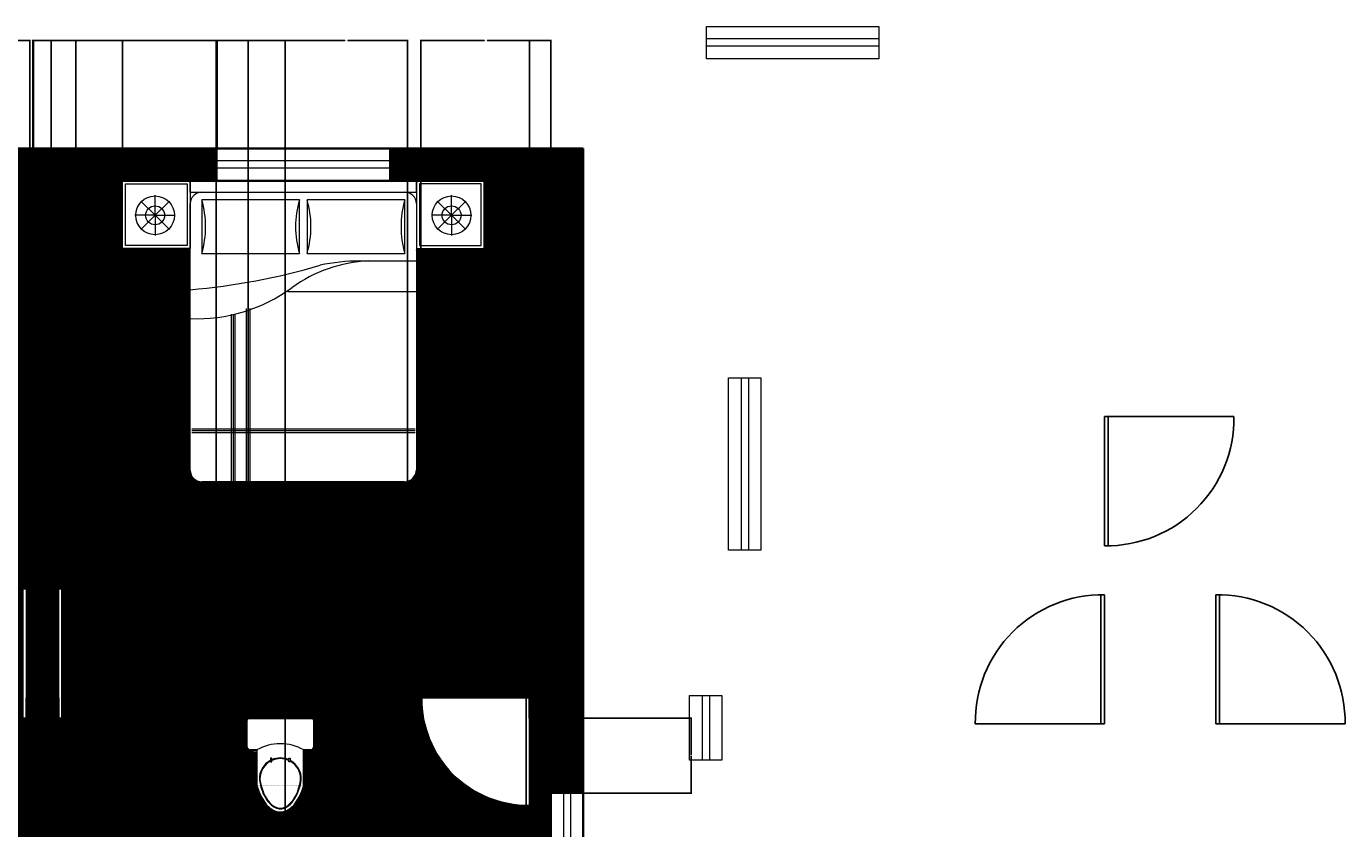
# Model space of a CAD drawing. Units: inches. Extents: x 205 to 1667, y -23 to 828.
# Tile 8 of 10: x 619 to 987, y 418 to 642. Entities that reach past the tile are written whole.
import ezdxf

# ---------------------------------------------------------------- set-up
doc = ezdxf.new("R2010")
doc.units = ezdxf.units.IN
doc.header["$MEASUREMENT"] = 0
for name, color, linetype, lineweight in [('A-ANNO-DIMS', 2, 'Continuous', 18), ('A-AREA-IDEN', 7, 'Continuous', 25), ('A-DOOR', 4, 'Continuous', 25), ('A-FLOR-FIXT', 9, 'Continuous', 18), ('A-FURN', 8, 'Continuous', 18), ('A-GLAZ', 4, 'Continuous', 18), ('A-WALL', 7, 'Continuous', 35)]:
    doc.layers.add(name, color=color, linetype=linetype, lineweight=lineweight)
doc.layers.add('A-FLOR-PATT', color=9, linetype='Continuous', lineweight=9, true_color=0xc7c8ca)
doc.styles.get("Standard").update_dxf_attribs({"font": 'arial.ttf'})
doc.dimstyles.get("Standard").update_dxf_attribs({"dimtxt": 0.18, "dimasz": 0.18, "dimexe": 0.18, "dimexo": 0.0625, "dimgap": 0.09, "dimtad": 0, "dimtih": 1, "dimtoh": 1, "dimdec": 4, "dimzin": 0, "dimdsep": 46, "dimtxsty": 'Standard', "dimcen": 0.09, "dimadec": 0, "dimazin": 0, "dimtfac": 1, "dimtdec": 4, "dimtofl": 0, "dimtmove": 0, "dimatfit": 3, "dimfxl": 1, "dimtolj": 1, "dimtzin": 0, "dimarcsym": 0})

# ---------------------------------------------------------------- blocks, each defined once
blk = doc.blocks.new('A$C068671E6')
for p, q in [((0, 1.5502), (0, 2.0002)), ((0, 2.0002), (0.45, 2.0002)), ((0.02, 1.5702), (0.02, 1.9802)), ((0.02, 1.9802), (0.43, 1.9802)), ((0.43, 1.9802), (0.43, 1.5702)), ((0.45, 2.0002), (0.45, 1.5502)), ((1.9506, 2.0002), (1.9506, 1.5502)), ((2.4006, 2.0002), (1.9506, 2.0002)), ((1.9706, 1.9802), (1.9706, 1.5702)), ((2.3806, 1.9802), (1.9706, 1.9802)), ((2.3806, 1.5702), (2.3806, 1.9802)), ((2.4006, 1.5502), (2.4006, 2.0002)), ((0.216, 1.7702), (0.121, 1.8652)), ((0.216, 1.7702), (0.216, 1.9046)), ((0.216, 1.7702), (0.3111, 1.8652)), ((2.1846, 1.7702), (2.0895, 1.8652)), ((2.1846, 1.7702), (2.1846, 1.9046)), ((2.1846, 1.7702), (2.2796, 1.8652)), ((0.216, 1.7702), (0.0817, 1.7702)), ((0.216, 1.7702), (0.121, 1.6752)), ((0.216, 1.7702), (0.216, 1.6358)), ((0.216, 1.7702), (0.3111, 1.6752)), ((0.216, 1.7702), (0.3504, 1.7702)), ((2.1846, 1.7702), (2.0502, 1.7702)), ((2.1846, 1.7702), (2.0895, 1.6752)), ((2.1846, 1.7702), (2.1846, 1.6358)), ((2.1846, 1.7702), (2.3189, 1.7702)), ((2.1846, 1.7702), (2.2796, 1.6752)), ((0.45, 1.5502), (0, 1.5502)), ((0.43, 1.5702), (0.02, 1.5702)), ((1.9506, 1.5502), (2.4006, 1.5502)), ((1.9706, 1.5702), (2.3806, 1.5702)), ((0.8202, 1.1507), (0.8202, 0)), ((0.8322, 1.1507), (0.8322, 0)), ((0.8442, 1.1507), (0.8442, 0)), ((0.722, 1.1146), (0.722, 0)), ((0.734, 1.1146), (0.734, 0)), ((0.746, 1.1146), (0.746, 0)), ((0.4599, 0.3521), (1.9437, 0.3521)), ((0.4599, 0.3401), (1.9437, 0.3401)), ((0.4599, 0.3281), (1.9437, 0.3281))]:
    blk.add_line(p, q)
at = {"linetype": 'ByBlock'}
for p, q in [((0.45, 1.924), (0.45, 2.0002)), ((0.45, 2.0002), (1.9506, 2.0002)), ((1.9506, 1.924), (1.9506, 2.0002)), ((0.45, 1.924), (1.9506, 1.924)), ((0.45, 0.0762), (0.45, 1.8478)), ((1.1744, 1.8732), (0.5262, 1.8732)), ((0.5262, 1.8732), (0.5262, 1.5176)), ((1.1744, 1.5176), (1.1744, 1.8732)), ((1.8744, 1.8732), (1.2252, 1.8732)), ((1.2252, 1.8732), (1.2252, 1.5176)), ((1.8744, 1.5176), (1.8744, 1.8732)), ((1.9506, 1.8478), (1.9506, 0.08)), ((0.5262, 1.5176), (1.1744, 1.5176)), ((1.2252, 1.5176), (1.8744, 1.5176)), ((1.5747, 1.4668), (1.9506, 1.4668)), ((1.0982, 1.2636), (1.9506, 1.2636)), ((1.8706, 0), (0.5262, 0))]:
    blk.add_line(p, q, dxfattribs=at)
for centre, radius in [((0.216, 1.7702), 0.1285), ((2.1846, 1.7702), 0.1285), ((0.216, 1.7702), 0.0628), ((2.1846, 1.7702), 0.0628)]:
    blk.add_circle(centre, radius)
for centre, radius, start, end in [((0.5262, 1.8478), 0.0762, 90, 180), ((-0.0834, 1.6954), 0.635, 343.73979, 16.26021), ((1.784, 1.6954), 0.635, 163.73979, 196.26021), ((0.6156, 1.6954), 0.635, 343.73979, 16.26021), ((2.484, 1.6954), 0.635, 163.73979, 196.26021), ((1.8744, 1.8478), 0.0762, 0, 90), ((0.0692, 5.6598), 4.4006, 274.96238, 286.39109), ((1.673, 0.534), 0.9338, 92.53978, 126.04031), ((1.5743, 0.2475), 1.2193, 89.98136, 102.46674), ((0.4931, 2.1535), 1.07, 267.6917, 306.10591), ((0.5262, 0.0762), 0.0762, 180, 270), ((1.8706, 0.08), 0.08, 270, 0)]:
    blk.add_arc(centre, radius, start, end, dxfattribs=at)
blk = doc.blocks.new('A$C0C6D4B22')
at = {"ltscale": 0.06}
for p, q in [((0.02, 0.73), (0.49, 0.73)), ((0, 0.5), (0, 0.71)), ((0.51, 0.71), (0.51, 0.5)), ((0.011, 0.465), (0.011, 0.469)), ((0.011, 0.469), (0.044, 0.469)), ((0.044, 0.462), (0.011, 0.465)), ((0.075, 0.48), (0.02, 0.48)), ((0.044, 0.469), (0.044, 0.478)), ((0.044, 0.478), (0.074, 0.478)), ((0.074, 0.462), (0.044, 0.462)), ((0.074, 0.478), (0.074, 0.462)), ((0.075, 0.206), (0.075, 0.48)), ((0.189, 0.415), (0.179, 0.415)), ((0.179, 0.415), (0.179, 0.388)), ((0.189, 0.388), (0.189, 0.415)), ((0.321, 0.388), (0.321, 0.415)), ((0.321, 0.415), (0.331, 0.415)), ((0.331, 0.415), (0.331, 0.388)), ((0.49, 0.48), (0.435, 0.48)), ((0.435, 0.206), (0.435, 0.48)), ((0.179, 0.388), (0.189, 0.388)), ((0.331, 0.388), (0.321, 0.388))]:
    blk.add_line(p, q, dxfattribs=at)
for centre, radius, start, end in [((0.02, 0.71), 0.02, 90, 180), ((0.49, 0.71), 0.02, 0, 90), ((0.255, 0.157), 0.37, 60.8534, 119.1466), ((0.02, 0.5), 0.02, 180, 270), ((0.255, 0.255), 0.162, 65.9871, 114.0129), ((0.255, 0.255), 0.157, 65.1738, 114.8262), ((0.49, 0.5), 0.02, 270, 0), ((0.255, 0.255), 0.162, 118.0804, 182.458), ((0.255, 0.255), 0.157, 119.0557, 202.516), ((0.255, 0.255), 0.162, 357.5995, 61.9196), ((0.255, 0.255), 0.157, 357.6909, 60.9443)]:
    blk.add_arc(centre, radius, start, end, dxfattribs=at)
blk.add_ellipse((0.255, 0.374), major_axis=(0, 0.374), ratio=0.539361, start_param=2.036707, end_param=4.246479, dxfattribs=at)
for points, knots in [([(0.093, 0.248), (0.105, 0.169), (0.136, 0.102), (0.2, 0.037), (0.228, 0.024), (0.255, 0.024), (0.288, 0.024), (0.324, 0.044), (0.384, 0.125), (0.408, 0.182), (0.417, 0.248)], [5.069811, 5.069811, 5.069811, 5.069811, 5.772291, 5.772291, 6.283185, 6.283185, 6.283185, 6.911741, 6.911741, 7.496594, 7.496594, 7.496594, 7.496594]), ([(0.11, 0.194), (0.119, 0.161), (0.132, 0.131), (0.18, 0.053), (0.22, 0.029), (0.291, 0.029), (0.33, 0.054), (0.386, 0.144), (0.404, 0.193), (0.412, 0.248)], [5.239766, 5.239766, 5.239766, 5.239766, 5.570281, 5.570281, 6.284782, 6.284782, 6.999284, 6.999284, 7.495839, 7.495839, 7.495839, 7.495839])]:
    blk.add_open_spline(points, degree=3, knots=knots, dxfattribs=at)
blk = doc.blocks.new('WIN-48IN')
for p, q in [((0, 0), (0, 9)), ((0, 9), (48, 9)), ((48, 9), (48, 0)), ((48, 5.5), (0, 5.5)), ((48, 3.5), (0, 3.5)), ((48, 0), (0, 0))]:
    blk.add_line(p, q)
blk = doc.blocks.new('WIN-BATH-18IN')
for p, q in [((0, 18), (9, 18)), ((0, 0), (0, 18)), ((3.5, 18), (3.5, 0)), ((5.5, 18), (5.5, 0)), ((9, 18), (9, 0)), ((9, 0), (0, 0))]:
    blk.add_line(p, q)
blk = doc.blocks.new('DOOR-SINGLE-36IN')
for p, q in [((35, 0), (35, 36)), ((36, 0), (36, 36)), ((35, 0), (36, 0))]:
    blk.add_line(p, q)
blk.add_arc((35.5, 0.5), 35.5, 89.1931, 180.8069)
blk = doc.blocks.new('DOOR-SINGLE-36IN-THRESHOLD')
for p, q in [((0, 0), (0, 36)), ((1, 0), (1, 36)), ((36, 0), (0, 0))]:
    blk.add_line(p, q)
blk.add_arc((0.5, 0.5), 35.5, 359.1931, 90.8069)
blk = doc.blocks.new('DOOR-SINGLE-30IN')
for p, q in [((30, 30), (0, 30)), ((0, 30), (0, 29)), ((30, 29), (0, 29))]:
    blk.add_line(p, q)
blk.add_arc((0.5, 29.5), 29.5, 269.029, 0.971)
blk = doc.blocks.new('*D24')
at = {"layer": 'A-ANNO-DIMS', "color": 0, "lineweight": -2, "transparency": 16777216}
for p, q in [((646.21, 514.72), (646.21, 499.51)), ((746.86, 514.72), (746.86, 499.51)), ((646.39, 499.69), (695.15, 499.69)), ((746.68, 499.69), (697.92, 499.69))]:
    blk.add_line(p, q, dxfattribs=at)
at = {"layer": 'A-ANNO-DIMS', "color": 0, "transparency": 16777216}
for points in [[(646.39, 499.72), (646.39, 499.66), (646.21, 499.69)], [(746.68, 499.72), (746.68, 499.66), (746.86, 499.69)]]:
    blk.add_solid(points, dxfattribs=at)
at = {"layer": 'Defpoints', "color": 0, "transparency": 16777216}
for p in [(646.21, 514.78), (746.86, 514.78), (746.86, 499.69)]:
    blk.add_point(p, dxfattribs=at)
at = {"layer": 'A-ANNO-DIMS', "color": 0, "transparency": 16777216, "insert": (696.53, 499.69), "char_height": 0.18, "attachment_point": 5}
blk.add_mtext('\\A1;BED GROUP 101 TYP.', dxfattribs=at)
blk = doc.blocks.new('*D25')
at = {"layer": 'A-ANNO-DIMS', "color": 0, "lineweight": -2, "transparency": 16777216}
for p, q in [((746.92, 598.65), (762.14, 598.65)), ((761.96, 598.47), (761.96, 556.9)), ((761.96, 514.96), (761.96, 556.54)), ((746.92, 514.78), (762.14, 514.78))]:
    blk.add_line(p, q, dxfattribs=at)
at = {"layer": 'A-ANNO-DIMS', "color": 0, "transparency": 16777216}
for points in [[(761.93, 598.47), (761.99, 598.47), (761.96, 598.65)], [(761.93, 514.96), (761.99, 514.96), (761.96, 514.78)]]:
    blk.add_solid(points, dxfattribs=at)
at = {"layer": 'Defpoints', "color": 0, "transparency": 16777216}
for p in [(746.86, 598.65), (761.96, 598.65), (746.86, 514.78)]:
    blk.add_point(p, dxfattribs=at)
at = {"layer": 'A-ANNO-DIMS', "color": 0, "transparency": 16777216, "insert": (761.96, 556.72), "char_height": 0.18, "attachment_point": 5}
blk.add_mtext('\\A1;84 TYP.', dxfattribs=at)
blk = doc.blocks.new('*D28')
at = {"layer": 'A-ANNO-DIMS', "color": 0, "lineweight": -2, "transparency": 16777216}
for p, q in [((583.31, 448.9), (583.31, 443.36)), ((619.44, 448.9), (619.44, 443.36)), ((583.49, 443.54), (600.01, 443.54)), ((619.26, 443.54), (602.73, 443.54))]:
    blk.add_line(p, q, dxfattribs=at)
at = {"layer": 'A-ANNO-DIMS', "color": 0, "transparency": 16777216}
for points in [[(583.49, 443.57), (583.49, 443.51), (583.31, 443.54)], [(619.26, 443.57), (619.26, 443.51), (619.44, 443.54)]]:
    blk.add_solid(points, dxfattribs=at)
at = {"layer": 'Defpoints', "color": 0, "transparency": 16777216}
for p in [(583.31, 448.96), (619.44, 448.96), (619.44, 443.54)]:
    blk.add_point(p, dxfattribs=at)
at = {"layer": 'A-ANNO-DIMS', "color": 0, "transparency": 16777216, "insert": (601.37, 443.54), "char_height": 0.18, "attachment_point": 5}
blk.add_mtext('\\A1;ROOM DOOR 36 TYP.', dxfattribs=at)
blk = doc.blocks.new('*D29')
at = {"layer": 'A-ANNO-DIMS', "color": 0, "lineweight": -2, "transparency": 16777216}
for p, q in [((619.5, 485.1), (625.04, 485.1)), ((624.86, 484.92), (624.86, 467.21)), ((624.86, 449.14), (624.86, 466.85)), ((619.5, 448.96), (625.04, 448.96))]:
    blk.add_line(p, q, dxfattribs=at)
at = {"layer": 'A-ANNO-DIMS', "color": 0, "transparency": 16777216}
for points in [[(624.83, 484.92), (624.89, 484.92), (624.86, 485.1)], [(624.83, 449.14), (624.89, 449.14), (624.86, 448.96)]]:
    blk.add_solid(points, dxfattribs=at)
at = {"layer": 'Defpoints', "color": 0, "transparency": 16777216}
for p in [(619.44, 485.1), (624.86, 485.1), (619.44, 448.96)]:
    blk.add_point(p, dxfattribs=at)
at = {"layer": 'A-ANNO-DIMS', "color": 0, "transparency": 16777216, "insert": (624.86, 467.03), "char_height": 0.18, "attachment_point": 5}
blk.add_mtext('\\A1;36 TYP.', dxfattribs=at)
blk = doc.blocks.new('*D30')
at = {"layer": 'A-ANNO-DIMS', "color": 0, "lineweight": -2, "transparency": 16777216}
for p, q in [((699.39, 449.15), (703.45, 449.15)), ((703.27, 448.97), (703.27, 436.17)), ((703.27, 423.01), (703.27, 435.8)), ((699.39, 422.83), (703.45, 422.83))]:
    blk.add_line(p, q, dxfattribs=at)
at = {"layer": 'A-ANNO-DIMS', "color": 0, "transparency": 16777216}
for points in [[(703.24, 448.97), (703.3, 448.97), (703.27, 449.15)], [(703.24, 423.01), (703.3, 423.01), (703.27, 422.83)]]:
    blk.add_solid(points, dxfattribs=at)
at = {"layer": 'Defpoints', "color": 0, "transparency": 16777216}
for p in [(699.32, 449.15), (703.27, 449.15), (699.32, 422.83)]:
    blk.add_point(p, dxfattribs=at)
at = {"layer": 'A-ANNO-DIMS', "color": 0, "transparency": 16777216, "insert": (703.27, 435.99), "char_height": 0.18, "attachment_point": 5}
blk.add_mtext('\\A1;WC 26 TYP.', dxfattribs=at)
blk = doc.blocks.new('*D31')
at = {"layer": 'A-ANNO-DIMS', "color": 0, "lineweight": -2, "transparency": 16777216}
for p, q in [((680.94, 422.76), (680.94, 418.7)), ((699.32, 422.76), (699.32, 418.7)), ((681.12, 418.88), (689.61, 418.88)), ((699.14, 418.88), (690.65, 418.88))]:
    blk.add_line(p, q, dxfattribs=at)
at = {"layer": 'A-ANNO-DIMS', "color": 0, "transparency": 16777216}
for points in [[(681.12, 418.91), (681.12, 418.85), (680.94, 418.88)], [(699.14, 418.91), (699.14, 418.85), (699.32, 418.88)]]:
    blk.add_solid(points, dxfattribs=at)
at = {"layer": 'Defpoints', "color": 0, "transparency": 16777216}
for p in [(680.94, 422.83), (699.32, 422.83), (699.32, 418.88)]:
    blk.add_point(p, dxfattribs=at)
at = {"layer": 'A-ANNO-DIMS', "color": 0, "transparency": 16777216, "insert": (690.13, 418.88), "char_height": 0.18, "attachment_point": 5}
blk.add_mtext('\\A1;18 TYP.', dxfattribs=at)
blk = doc.blocks.new('*D47')
at = {"layer": 'A-ANNO-DIMS', "color": 0, "lineweight": -2, "transparency": 16777216}
for p, q in [((569.57, 607.71), (569.57, 637.89)), ((569.75, 637.71), (620.6, 637.71)), ((672.35, 637.71), (621.51, 637.71)), ((672.53, 607.71), (672.53, 637.89))]:
    blk.add_line(p, q, dxfattribs=at)
at = {"layer": 'A-ANNO-DIMS', "color": 0, "transparency": 16777216}
for points in [[(569.75, 637.74), (569.75, 637.68), (569.57, 637.71)], [(672.35, 637.74), (672.35, 637.68), (672.53, 637.71)]]:
    blk.add_solid(points, dxfattribs=at)
at = {"layer": 'Defpoints', "color": 0, "transparency": 16777216}
for p in [(672.53, 637.71), (569.57, 607.65), (672.53, 607.65)]:
    blk.add_point(p, dxfattribs=at)
at = {"layer": 'A-ANNO-DIMS', "color": 0, "transparency": 16777216, "insert": (621.05, 637.71), "char_height": 0.18, "attachment_point": 5}
blk.add_mtext('\\A1;102.96', dxfattribs=at)
blk = doc.blocks.new('*D49')
at = {"layer": 'A-ANNO-DIMS', "color": 0, "lineweight": -2, "transparency": 16777216}
for p, q in [((765.49, 448.96), (804.67, 448.96)), ((804.49, 448.78), (804.49, 438.69)), ((804.49, 428.24), (804.49, 438.33)), ((765.49, 428.06), (804.67, 428.06))]:
    blk.add_line(p, q, dxfattribs=at)
at = {"layer": 'A-ANNO-DIMS', "color": 0, "transparency": 16777216}
for points in [[(804.46, 448.78), (804.52, 448.78), (804.49, 448.96)], [(804.46, 428.24), (804.52, 428.24), (804.49, 428.06)]]:
    blk.add_solid(points, dxfattribs=at)
at = {"layer": 'Defpoints', "color": 0, "transparency": 16777216}
for p in [(765.43, 448.96), (765.43, 428.06), (804.49, 428.06)]:
    blk.add_point(p, dxfattribs=at)
at = {"layer": 'A-ANNO-DIMS', "color": 0, "transparency": 16777216, "insert": (804.49, 438.51), "char_height": 0.18, "attachment_point": 5}
blk.add_mtext('\\A1;20.903', dxfattribs=at)
blk = doc.blocks.new('*D54')
at = {"layer": 'A-ANNO-DIMS', "color": 0, "lineweight": -2, "transparency": 16777216}
for p, q in [((729.22, 16.71), (729.22, 637.89)), ((729.4, 637.71), (746.95, 637.71)), ((765.25, 637.71), (747.7, 637.71)), ((765.43, 16.71), (765.43, 637.89))]:
    blk.add_line(p, q, dxfattribs=at)
at = {"layer": 'A-ANNO-DIMS', "color": 0, "transparency": 16777216}
for points in [[(729.4, 637.74), (729.4, 637.68), (729.22, 637.71)], [(765.25, 637.74), (765.25, 637.68), (765.43, 637.71)]]:
    blk.add_solid(points, dxfattribs=at)
at = {"layer": 'Defpoints', "color": 0, "transparency": 16777216}
for p in [(729.22, 637.71), (729.22, 16.65), (765.43, 16.65)]:
    blk.add_point(p, dxfattribs=at)
at = {"layer": 'A-ANNO-DIMS', "color": 0, "transparency": 16777216, "insert": (747.33, 637.71), "char_height": 0.18, "attachment_point": 5}
blk.add_mtext('\\A1;36.21', dxfattribs=at)
blk = doc.blocks.new('*D55')
at = {"layer": 'A-ANNO-DIMS', "color": 0, "lineweight": -2, "transparency": 16777216}
for p, q in [((621.22, 16.71), (621.22, 637.89)), ((621.4, 637.71), (627.01, 637.71)), ((633.04, 637.71), (627.43, 637.71)), ((633.22, 16.71), (633.22, 637.89))]:
    blk.add_line(p, q, dxfattribs=at)
at = {"layer": 'A-ANNO-DIMS', "color": 0, "transparency": 16777216}
for points in [[(621.4, 637.74), (621.4, 637.68), (621.22, 637.71)], [(633.04, 637.74), (633.04, 637.68), (633.22, 637.71)]]:
    blk.add_solid(points, dxfattribs=at)
at = {"layer": 'Defpoints', "color": 0, "transparency": 16777216}
for p in [(633.22, 637.71), (621.22, 16.65), (633.22, 16.65)]:
    blk.add_point(p, dxfattribs=at)
at = {"layer": 'A-ANNO-DIMS', "color": 0, "transparency": 16777216, "insert": (627.22, 637.71), "char_height": 0.18, "attachment_point": 5}
blk.add_mtext('\\A1;12', dxfattribs=at)
blk = doc.blocks.new('*D58')
at = {"layer": 'A-ANNO-DIMS', "color": 0, "lineweight": -2, "transparency": 16777216}
for p, q in [((759.53, 454.71), (759.53, 637.89)), ((759.71, 637.71), (762.1, 637.71)), ((765.25, 637.71), (762.86, 637.71)), ((765.43, 454.71), (765.43, 637.89))]:
    blk.add_line(p, q, dxfattribs=at)
at = {"layer": 'A-ANNO-DIMS', "color": 0, "transparency": 16777216}
for points in [[(759.71, 637.74), (759.71, 637.68), (759.53, 637.71)], [(765.25, 637.74), (765.25, 637.68), (765.43, 637.71)]]:
    blk.add_solid(points, dxfattribs=at)
at = {"layer": 'Defpoints', "color": 0, "transparency": 16777216}
for p in [(765.43, 637.71), (759.53, 454.65), (765.43, 454.65)]:
    blk.add_point(p, dxfattribs=at)
at = {"layer": 'A-ANNO-DIMS', "color": 0, "transparency": 16777216, "insert": (762.48, 637.71), "char_height": 0.18, "attachment_point": 5}
blk.add_mtext('\\A1;5.901', dxfattribs=at)
blk = doc.blocks.new('*D62')
at = {"layer": 'A-ANNO-DIMS', "color": 0, "lineweight": -2, "transparency": 16777216}
for p, q in [((672.3, 449.03), (672.3, 637.89)), ((672.48, 637.71), (676.33, 637.71)), ((680.97, 637.71), (677.12, 637.71)), ((681.15, 449), (681.15, 637.89))]:
    blk.add_line(p, q, dxfattribs=at)
at = {"layer": 'A-ANNO-DIMS', "color": 0, "transparency": 16777216}
for points in [[(672.48, 637.74), (672.48, 637.68), (672.3, 637.71)], [(680.97, 637.74), (680.97, 637.68), (681.15, 637.71)]]:
    blk.add_solid(points, dxfattribs=at)
at = {"layer": 'Defpoints', "color": 0, "transparency": 16777216}
for p in [(681.15, 637.71), (672.3, 448.96), (681.15, 448.94)]:
    blk.add_point(p, dxfattribs=at)
at = {"layer": 'A-ANNO-DIMS', "color": 0, "transparency": 16777216, "insert": (676.72, 637.71), "char_height": 0.18, "attachment_point": 5}
blk.add_mtext('\\A1;8.844', dxfattribs=at)
blk = doc.blocks.new('*D66')
at = {"layer": 'A-ANNO-DIMS', "color": 0, "lineweight": -2, "transparency": 16777216}
for p, q in [((691.51, 243.5), (691.51, 637.89)), ((691.69, 637.71), (708.11, 637.71)), ((725.32, 637.71), (708.9, 637.71)), ((725.5, 243.5), (725.5, 637.89))]:
    blk.add_line(p, q, dxfattribs=at)
at = {"layer": 'A-ANNO-DIMS', "color": 0, "transparency": 16777216}
for points in [[(691.69, 637.74), (691.69, 637.68), (691.51, 637.71)], [(725.32, 637.74), (725.32, 637.68), (725.5, 637.71)]]:
    blk.add_solid(points, dxfattribs=at)
at = {"layer": 'Defpoints', "color": 0, "transparency": 16777216}
for p in [(725.5, 637.71), (691.51, 243.44), (725.5, 243.44)]:
    blk.add_point(p, dxfattribs=at)
at = {"layer": 'A-ANNO-DIMS', "color": 0, "transparency": 16777216, "insert": (708.5, 637.71), "char_height": 0.18, "attachment_point": 5}
blk.add_mtext('\\A1;33.99', dxfattribs=at)
blk = doc.blocks.new('*D68')
at = {"layer": 'A-ANNO-DIMS', "color": 0, "lineweight": -2, "transparency": 16777216}
for p, q in [((626.35, 153.44), (626.35, 637.89)), ((626.53, 637.71), (658.53, 637.71)), ((691.33, 637.71), (659.32, 637.71)), ((691.51, 177.11), (691.51, 637.89))]:
    blk.add_line(p, q, dxfattribs=at)
at = {"layer": 'A-ANNO-DIMS', "color": 0, "transparency": 16777216}
for points in [[(626.53, 637.74), (626.53, 637.68), (626.35, 637.71)], [(691.33, 637.74), (691.33, 637.68), (691.51, 637.71)]]:
    blk.add_solid(points, dxfattribs=at)
at = {"layer": 'Defpoints', "color": 0, "transparency": 16777216}
for p in [(626.35, 637.71), (691.51, 177.05), (626.35, 153.38)]:
    blk.add_point(p, dxfattribs=at)
at = {"layer": 'A-ANNO-DIMS', "color": 0, "transparency": 16777216, "insert": (658.93, 637.71), "char_height": 0.18, "attachment_point": 5}
blk.add_mtext('\\A1;65.16', dxfattribs=at)
blk = doc.blocks.new('*D73')
at = {"layer": 'A-ANNO-DIMS', "color": 0, "lineweight": -2, "transparency": 16777216}
for p, q in [((626.35, 598.71), (626.35, 637.89)), ((626.53, 637.71), (635.89, 637.71)), ((646.03, 637.71), (636.66, 637.71)), ((646.21, 598.71), (646.21, 637.89))]:
    blk.add_line(p, q, dxfattribs=at)
at = {"layer": 'A-ANNO-DIMS', "color": 0, "transparency": 16777216}
for points in [[(626.53, 637.74), (626.53, 637.68), (626.35, 637.71)], [(646.03, 637.74), (646.03, 637.68), (646.21, 637.71)]]:
    blk.add_solid(points, dxfattribs=at)
at = {"layer": 'Defpoints', "color": 0, "transparency": 16777216}
for p in [(646.21, 637.71), (626.35, 598.65), (646.21, 598.65)]:
    blk.add_point(p, dxfattribs=at)
at = {"layer": 'A-ANNO-DIMS', "color": 0, "transparency": 16777216, "insert": (636.28, 637.71), "char_height": 0.18, "attachment_point": 5}
blk.add_mtext('\\A1;19.86', dxfattribs=at)
blk = doc.blocks.new('*D80')
at = {"layer": 'A-ANNO-DIMS', "color": 0, "lineweight": -2, "transparency": 16777216}
for p, q in [((596.44, 213.99), (596.44, 637.89)), ((596.62, 637.71), (608.22, 637.71)), ((620.26, 637.71), (608.66, 637.71)), ((620.44, 213.99), (620.44, 637.89))]:
    blk.add_line(p, q, dxfattribs=at)
at = {"layer": 'A-ANNO-DIMS', "color": 0, "transparency": 16777216}
for points in [[(596.62, 637.74), (596.62, 637.68), (596.44, 637.71)], [(620.26, 637.74), (620.26, 637.68), (620.44, 637.71)]]:
    blk.add_solid(points, dxfattribs=at)
at = {"layer": 'Defpoints', "color": 0, "transparency": 16777216}
for p in [(596.44, 637.71), (596.44, 213.93), (620.44, 213.93)]:
    blk.add_point(p, dxfattribs=at)
at = {"layer": 'A-ANNO-DIMS', "color": 0, "transparency": 16777216, "insert": (608.44, 637.71), "char_height": 0.18, "attachment_point": 5}
blk.add_mtext('\\A1;24', dxfattribs=at)
blk = doc.blocks.new('*D87')
at = {"layer": 'A-ANNO-DIMS', "color": 0, "lineweight": -2, "transparency": 16777216}
for p, q in [((621.44, 598.71), (621.44, 637.89)), ((621.62, 637.71), (623.5, 637.71)), ((626.17, 637.71), (624.29, 637.71)), ((626.35, 598.71), (626.35, 637.89))]:
    blk.add_line(p, q, dxfattribs=at)
at = {"layer": 'A-ANNO-DIMS', "color": 0, "transparency": 16777216}
for points in [[(621.62, 637.74), (621.62, 637.68), (621.44, 637.71)], [(626.17, 637.74), (626.17, 637.68), (626.35, 637.71)]]:
    blk.add_solid(points, dxfattribs=at)
at = {"layer": 'Defpoints', "color": 0, "transparency": 16777216}
for p in [(626.35, 637.71), (621.44, 598.65), (626.35, 598.65)]:
    blk.add_point(p, dxfattribs=at)
at = {"layer": 'A-ANNO-DIMS', "color": 0, "transparency": 16777216, "insert": (623.89, 637.71), "char_height": 0.18, "attachment_point": 5}
blk.add_mtext('\\A1;4.906', dxfattribs=at)

msp = doc.modelspace()

# ---------------------------------------------------------------- hatches: boundary and pattern name
at = {"layer": 'A-FLOR-PATT'}
h = msp.add_hatch(dxfattribs=at)
h.set_pattern_fill('ANSI31', color=256)
h.paths.add_polyline_path([(774.4305, 607.6511), (720.5338, 607.6511), (720.5338, 598.6511), (727.9933, 598.6511), (746.8614, 598.6511), (765.4305, 598.6511), (765.4305, 454.6511), (759.5298, 454.6511), (759.5298, 448.9635), (765.4305, 448.9635), (765.4305, 428.0602), (774.4305, 428.0602)])
h.paths.add_polyline_path([(765.4305, 598.6511), (746.8614, 598.6511), (746.8614, 579.7829), (727.9933, 579.7829), (727.9933, 518.1387, -0.41421701), (724.6389, 514.7843), (668.2693, 514.7843, -0.41421356), (665.0743, 517.9793), (665.0743, 579.7829), (646.2062, 579.7829), (646.2062, 598.6511), (626.3468, 598.6511), (626.3468, 454.6511), (628.3468, 454.6511), (628.3468, 484.9635, -0.41421356), (664.3468, 449.9635), (664.3468, 454.6511), (729.3305, 454.6511), (758.5298, 454.6511), (759.5298, 454.6511), (765.4305, 454.6511)])
h.paths.add_polyline_path([(621.4404, 598.6511), (471.4305, 598.6511), (471.4305, 568.8442), (490.2987, 568.8442), (490.2987, 549.9761), (551.9429, 549.9761, -0.41421701), (555.2973, 546.6217), (555.2973, 490.2521, -0.41421356), (552.1023, 487.0571), (490.2987, 487.0571), (490.2987, 468.189), (471.4305, 468.189), (471.4305, 454.6511), (583.4404, 454.6511), (583.4404, 449.9635, -0.41421356), (619.4404, 484.9635), (619.4404, 454.6511), (621.4404, 454.6511)])
h.paths.add_polyline_path([(672.5338, 607.6511), (569.5707, 607.6511), (569.5707, 598.6511), (621.4404, 598.6511), (621.4404, 454.6511), (619.4404, 454.6511), (619.4404, 448.9635), (628.3468, 448.9635), (628.3468, 454.6511), (626.3468, 454.6511), (626.3468, 598.6511), (646.2062, 598.6511), (665.0743, 598.6511), (672.5338, 598.6511)])
h.paths.add_polyline_path([(521.5707, 607.6511), (462.4305, 607.6511), (462.4305, 407.4306), (471.4305, 407.4306), (471.4305, 448.9635), (583.4404, 448.9635, -0.0070419), (583.4404, 449.9635), (583.4404, 454.6511), (471.4305, 454.6511), (471.4305, 468.189), (471.4305, 487.0571), (471.4305, 549.9761), (471.4305, 568.8442), (471.4305, 598.6511), (521.5707, 598.6511)])
h.paths.add_polyline_path([(471.4305, 314.3187), (583.4404, 314.3187), (583.4404, 319.9388), (471.4305, 319.9388), (471.4305, 359.4306), (462.4305, 359.4306), (462.4305, 7.6511), (471.4305, 7.6511), (471.4305, 204.9321), (521.9355, 204.9321), (521.9355, 213.9321), (471.4305, 213.9321)])
h.paths.add_polyline_path([(774.4305, 410.0602), (765.4305, 410.0602), (765.4305, 389.1569), (672.3024, 389.1569), (672.3024, 448.9635), (681.1739, 448.9635, -0.18532444), (681.6564, 449.1487), (698.6035, 449.1487), (729.3305, 448.9635), (729.3305, 454.6511), (664.3468, 454.6511), (664.3468, 449.9635, -0.0070419), (664.3468, 448.9635), (666.3024, 448.9635), (666.3024, 378.2485), (672.3024, 378.2485), (672.3024, 383.1306), (765.4305, 383.1306), (765.4305, 360.5347), (774.4305, 360.5347)])
h.paths.add_polyline_path([(774.4305, 342.5347), (765.4305, 342.5347), (765.4305, 319.9388), (672.3024, 319.9388), (672.3024, 348.5574), (671.0896, 348.5574, -0.04071533), (666.3024, 348.2485), (666.3024, 319.9388), (664.3468, 319.9388, -0.0070419), (664.3468, 318.9388), (664.3468, 314.3187), (765.4305, 314.3187), (765.4305, 290.8426), (774.4305, 290.8426)])
h.paths.add_polyline_path([(774.4305, 242.8426), (765.4305, 242.8426), (765.4305, 104.6382), (626.3468, 104.6382), (626.3468, 110.5917), (617.3468, 110.5917), (617.3468, 95.6382), (765.4305, 95.6382), (765.4305, 16.6511), (621.2232, 16.6511), (621.2232, 7.6511), (774.4305, 7.6511)])
h.paths.add_polyline_path([(626.3468, 314.3187), (628.3468, 314.3187), (628.3468, 319.9388), (619.4404, 319.9388), (619.4404, 314.3187), (620.4404, 314.3187), (620.4404, 213.9321), (569.9355, 213.9321), (569.9355, 204.9321), (617.3468, 204.9321), (617.3468, 153.3751), (626.3468, 153.3751)])
h.paths.add_polyline_path([(620.4404, 314.3187), (619.4404, 314.3187), (619.4404, 319.9388), (628.3468, 319.9388), (629.3468, 319.9388), (629.3468, 283.9388, 0.40598745), (664.3468, 318.9388), (664.3468, 319.9388), (666.3024, 319.9388), (666.3024, 348.2485), (666.3024, 377.2485), (666.3024, 378.2485), (666.3024, 448.9635), (664.3468, 448.9635), (664.3468, 449.9635, 0.40598745), (629.3468, 484.9635), (629.3468, 448.9635), (628.3468, 448.9635), (619.4404, 448.9635), (618.4404, 448.9635), (618.4404, 484.9635, 0.40598745), (583.4404, 449.9635), (583.4404, 448.9635), (471.4305, 448.9635), (471.4305, 407.4306), (471.4305, 359.4306), (471.4305, 319.9388), (583.4404, 319.9388), (583.4404, 314.3187), (495.4305, 314.3187), (495.4305, 237.9321), (620.4404, 237.9321)])
h.paths.add_polyline_path([(525.0876, 347.7863), (513.5657, 347.7863), (512.0216, 362.1672), (526.6317, 362.1672)], flags=16)
h.paths.add_polyline_path([(550.9499, 370.1471), (536.569, 368.6029), (536.569, 383.2131), (550.9499, 381.6689)], flags=16)
h.paths.add_polyline_path([(530.7713, 364.5431), (508.0415, 364.5431, -0.41421356), (504.7944, 367.7902), (504.7944, 403.5085, -0.41421356), (508.0415, 406.7556), (530.7713, 406.7556, -0.41421356), (534.0184, 403.5085), (534.0184, 367.7902, -0.41421356)], flags=16)
h.paths.add_polyline_path([(550.9499, 389.6298), (536.569, 388.0856), (536.569, 402.6958), (550.9499, 401.1516)], flags=16)
h.paths.add_polyline_path([(502.2439, 368.6029), (487.863, 370.1471), (487.863, 381.6689), (502.2439, 383.2131)], flags=16)
h.paths.add_polyline_path([(502.2439, 388.0856), (487.863, 389.6298), (487.863, 401.1516), (502.2439, 402.6958)], flags=16)
h.paths.add_polyline_path([(526.6317, 409.1315), (512.0216, 409.1315), (513.5657, 423.5124), (525.0876, 423.5124)], flags=16)
h.paths.add_polyline_path([(765.4305, 290.8426), (765.4305, 314.3187), (664.3468, 314.3187), (664.3468, 318.9388, -0.41421356), (628.3468, 283.9388), (628.3468, 314.3187), (626.3468, 314.3187), (626.3468, 153.3751), (638.3468, 153.3751, -0.4196361), (617.5748, 131.9834, -0.4196361), (638.3468, 110.5917), (626.3468, 110.5917), (626.3468, 104.6382), (765.4305, 104.6382), (765.4305, 242.8426)])
h.paths.add_polyline_path([(691.5064, 243.4363), (693.2483, 243.4363), (725.4984, 243.4363), (725.4984, 241.7329), (725.4984, 177.0512), (723.7564, 177.0512), (691.5064, 177.0512), (691.5064, 178.7545)], flags=16)
h.paths.add_polyline_path([(689.8658, 265.2977), (689.8658, 296.6873, -0.41421356), (690.8346, 297.6561), (724.6111, 297.6561, -0.41421356), (725.5799, 296.6873), (725.5799, 265.2977, -0.41421356), (724.6111, 264.3289), (690.8346, 264.3289, -0.41421356)], flags=16)
h.paths.add_polyline_path([(694.1286, 265.6852), (694.1286, 288.9368, -0.41421356), (695.0974, 289.9056), (720.3483, 289.9056, -0.41421356), (721.3171, 288.9368), (721.3171, 265.6852, -0.04533947), (721.3013, 265.5106, -0.3531705), (720.3282, 264.7164), (695.0974, 264.7164, -0.41421356)], flags=0)
h.paths.add_polyline_path([(694.1286, 291.2619), (694.1286, 294.7497, -0.41421356), (695.0974, 295.7185), (720.3483, 295.7185, -0.41421356), (721.3171, 294.7497), (721.3171, 291.2619, -0.41421356), (720.3483, 290.2931), (695.0974, 290.2931, -0.41421356)], flags=0)
h.paths.add_polyline_path([(734.4369, 244.6615, -0.41421356), (735.2682, 245.4928), (762.2019, 245.4928, -0.41421356), (763.0332, 244.6615), (763.0332, 168.183, -0.41421356), (762.2019, 167.3517), (735.2682, 167.3517, -0.41421356), (734.4369, 168.183)], flags=16)
h.paths.add_polyline_path([(761.7032, 242.1676), (761.7032, 170.6768), (735.6007, 171.0093, -0.41421356), (734.7694, 171.8406), (734.7694, 193.5102, -0.56972741), (735.6007, 194.674, -0.41421356), (734.7694, 195.5053), (734.7694, 217.3423, -0.56972741), (735.6007, 218.5061, -0.41421356), (734.7694, 219.3374), (734.7694, 241.0038, -0.41421356), (735.6007, 241.8351), (735.1643, 242.1676)], flags=16)
h.paths.add_polyline_path([(757.5467, 171.0093), (760.5393, 171.0093, 0.41421356), (761.3706, 171.8406), (761.3706, 193.5102, 0.41421356), (760.5393, 194.3415), (757.5467, 194.3415, 0.41421356), (756.7154, 193.5102), (756.7155, 171.8534, 0.41871477)], flags=0)
h.paths.add_polyline_path([(756.7154, 241.0038, -0.41421356), (757.5467, 241.8351), (760.5393, 241.8351, -0.41421356), (761.3706, 241.0038), (761.3706, 219.3374, -0.41421356), (760.5393, 218.5061), (760.5393, 218.1736, -0.41421356), (761.3706, 217.3423), (761.3706, 195.5053, -0.41421356), (760.5393, 194.674), (757.5467, 194.674, -0.56972741), (756.3829, 195.5053, -0.41421356), (755.5516, 194.674), (755.5516, 194.3415, -0.41421356), (756.3829, 193.5102), (756.7154, 171.8406), (756.3829, 193.5102, 0.41421356), (755.5516, 194.3415), (735.6007, 194.674), (755.5516, 194.674, 0.41421356), (756.3829, 195.5053), (756.3829, 217.3423, 0.41421356), (755.5516, 218.1736), (735.6007, 218.5061), (755.5516, 218.5061, 0.41421356), (756.3829, 219.3374)], flags=0)
h.paths.add_polyline_path([(694.5151, 150.3608), (728.2916, 150.3608, -0.41421356), (729.2604, 149.3919), (729.2604, 118.0023, -0.41421356), (728.2916, 117.0335), (694.5151, 117.0335, -0.41421356), (693.5463, 118.0023), (693.5463, 149.3919, -0.41421356)], flags=16)
h.paths.add_polyline_path([(724.0288, 149.9732, -0.41421356), (724.9977, 149.0044), (724.9977, 125.7529, -0.41421356), (724.0288, 124.784), (698.7779, 124.784, -0.41421356), (697.8091, 125.7529), (697.8091, 149.0044, -0.04533947), (697.825, 149.179, -0.3531705), (698.798, 149.9732)], flags=0)
h.paths.add_polyline_path([(698.7779, 124.3965), (724.0288, 124.3965, -0.41421356), (724.9977, 123.4277), (724.9977, 119.94, -0.41421356), (724.0288, 118.9711), (698.7779, 118.9711, -0.41421356), (697.8091, 119.94), (697.8091, 123.4277, -0.41421356)], flags=0)
h = msp.add_hatch(dxfattribs=at)
h.set_pattern_fill('ANSI31', color=256)
edge = h.paths.add_edge_path()
edge.add_line((729.5256, 454.1511), (729.3305, 448.9635))
edge.add_line((729.3305, 448.9635), (699.086, 448.9635))
edge.add_arc((698.6035, 448.4276), 0.7212, 0, 48.002211, ccw=False)
edge.add_line((699.3246, 448.4276), (699.3246, 440.8555))
edge.add_arc((698.6035, 440.8555), 0.7212, -90, 0, ccw=False)
edge.add_line((698.6035, 440.1343), (696.6203, 440.1343))
edge.add_line((696.6203, 440.1343), (696.6203, 430.2456))
edge.add_ellipse((690.1299, 436.2963), major_axis=(0, 13.4691), ratio=0.53936076, start_angle=132.992596, end_angle=227.007404, ccw=False)
edge.add_line((683.6396, 430.2456), (683.6396, 439.4922))
edge.add_line((683.6396, 439.4922), (682.5343, 439.4922))
edge.add_line((682.5343, 439.4922), (681.3419, 439.5773))
edge.add_line((681.3419, 439.5773), (681.3419, 439.7207))
edge.add_line((681.3419, 439.7207), (682.5343, 439.7207))
edge.add_line((682.5343, 439.7207), (682.5343, 440.1343))
edge.add_line((682.5343, 440.1343), (681.6564, 440.1343))
edge.add_arc((681.6564, 440.8555), 0.7212, 180.001025, 270, ccw=False)
edge.add_line((680.9353, 440.8555), (680.9353, 448.4276))
edge.add_arc((681.6564, 448.4276), 0.7212, 131.997789, 180.001025, ccw=False)
edge.add_line((681.1739, 448.9635), (672.3024, 448.9635))
edge.add_line((672.3024, 448.9635), (672.3024, 389.1569))
edge.add_line((672.3024, 389.1569), (765.4305, 389.1569))
edge.add_line((765.4305, 389.1569), (765.4305, 448.9635))
edge.add_line((765.4305, 448.9635), (759.5298, 448.9635))
edge.add_line((759.5298, 448.9635), (759.5298, 424.6511))
edge.add_arc((759.0298, 454.1511), 29.5042, 180, 270.971022, ccw=False)
edge = h.paths.add_edge_path()
edge.add_line((765.4305, 383.1306), (672.3024, 383.1306))
edge.add_line((672.3024, 383.1306), (672.3024, 378.2485))
edge.add_line((672.3024, 378.2485), (696.3024, 378.2485))
edge.add_arc((666.8024, 377.7485), 29.5042, -81.644907, 0.971022, ccw=False)
edge.add_line((671.0896, 348.5574), (672.3024, 348.5574))
edge.add_line((672.3024, 348.5574), (672.3024, 319.9388))
edge.add_line((672.3024, 319.9388), (736.1952, 319.9388))
edge.add_arc((736.1952, 320.6599), 0.7212, 180, 270.001025, ccw=False)
edge.add_line((735.474, 320.6599), (735.474, 328.232))
edge.add_arc((736.1952, 328.232), 0.7212, 90, 180, ccw=False)
edge.add_line((736.1952, 328.9532), (738.1783, 328.9532))
edge.add_line((738.1783, 328.9532), (738.1783, 338.8419))
edge.add_ellipse((744.6687, 332.7911), major_axis=(0, 13.4691), ratio=0.53936076, start_angle=-47.007404, end_angle=47.007404, ccw=False)
edge.add_line((751.1591, 338.8419), (751.1591, 329.5953))
edge.add_line((751.1591, 329.5953), (752.2643, 329.5953))
edge.add_line((752.2643, 329.5953), (753.4567, 329.5102))
edge.add_line((753.4567, 329.5102), (753.4567, 329.3668))
edge.add_line((753.4567, 329.3668), (752.2643, 329.3668))
edge.add_line((752.2643, 329.3668), (752.2643, 328.9532))
edge.add_line((752.2643, 328.9532), (753.1422, 328.9532))
edge.add_arc((753.1422, 328.232), 0.7212, 0.001025, 90, ccw=False)
edge.add_line((753.8634, 328.232), (753.8634, 320.6599))
edge.add_arc((753.1422, 320.6599), 0.7212, -89.998975, 0.001025, ccw=False)
edge.add_line((753.1422, 319.9388), (765.4305, 319.9388))
edge.add_line((765.4305, 319.9388), (765.4305, 383.1306))

# ---------------------------------------------------------------- linework, layer by layer
at = {"layer": 'A-DOOR'}
msp.add_line((729.3305, 454.6511), (758.5298, 454.6511), dxfattribs=at)
at = {"layer": 'A-WALL'}
for p, q in [((774.4305, 607.6511), (462.4305, 607.6511)), ((774.4305, 7.6511), (774.4305, 607.6511)), ((621.4404, 598.6511), (471.4305, 598.6511)), ((621.4404, 598.6511), (621.4404, 454.6511)), ((765.4305, 598.6511), (626.3468, 598.6511)), ((626.3468, 598.6511), (626.3468, 454.6511)), ((765.4305, 454.6511), (765.4305, 598.6511)), ((621.4404, 454.6511), (619.4404, 454.6511)), ((619.4404, 448.9635), (619.4404, 454.6511)), ((628.3468, 454.6511), (626.3468, 454.6511)), ((628.3468, 454.6511), (628.3468, 448.9635)), ((664.3468, 454.6511), (664.3468, 448.9635)), ((729.3305, 454.6511), (664.3468, 454.6511)), ((729.3305, 454.6511), (729.3305, 448.9635)), ((765.4305, 454.6511), (759.5298, 454.6511)), ((759.5298, 454.6511), (759.5298, 448.9635)), ((628.3468, 448.9635), (619.4404, 448.9635)), ((666.3024, 448.9635), (664.3468, 448.9635)), ((666.3024, 378.2485), (666.3024, 448.9635)), ((672.3024, 389.1569), (672.3024, 448.9635)), ((729.3305, 448.9635), (672.3024, 448.9635)), ((765.4305, 448.9635), (759.5298, 448.9635)), ((765.4305, 389.1569), (765.4305, 448.9635))]:
    msp.add_line(p, q, dxfattribs=at)

# ---------------------------------------------------------------- block references
at = {"layer": 'A-DOOR', "extrusion": (0, 0, -1), "zscale": -1, "rotation": 180}
msp.add_blockref('DOOR-SINGLE-36IN-THRESHOLD', (-919.5788, 532.9463), dxfattribs=at)
at = {"layer": 'A-DOOR'}
for name, p in [('DOOR-SINGLE-36IN', (583.44, 448.964)), ('DOOR-SINGLE-36IN-THRESHOLD', (950.539, 447.329))]:
    msp.add_blockref(name, p, dxfattribs=at)
at = {"layer": 'A-DOOR', "extrusion": (0, 0, -1), "zscale": -1}
for name, p in [('DOOR-SINGLE-36IN', (-664.3472, 448.964)), ('DOOR-SINGLE-36IN-THRESHOLD', (-919.5782, 447.329))]:
    msp.add_blockref(name, p, dxfattribs=at)
at = {"layer": 'A-DOOR', "rotation": 270.0000000000002}
msp.add_blockref('DOOR-SINGLE-30IN', (729.5293, 454.6515), dxfattribs=at)
at = {"layer": 'A-FLOR-FIXT', "xscale": 36.0575823356732, "yscale": 36.0575823356732, "zscale": 36.0575823356732}
msp.add_blockref('A$C0C6D4B22', (680.9353, 422.8273), dxfattribs=at)
at = {"layer": 'A-FURN', "xscale": 41.92918703190525, "yscale": 41.92918703190525, "zscale": 41.92918703190525}
msp.add_blockref('A$C068671E6', (646.2062, 514.7843), dxfattribs=at)
at = {"layer": 'A-GLAZ'}
for name, p in [('WIN-48IN', (808.7257, 632.6367)), ('WIN-48IN', (672.534, 598.651)), ('WIN-BATH-18IN', (804.053, 437.2226)), ('WIN-BATH-18IN', (765.431, 410.06))]:
    msp.add_blockref(name, p, dxfattribs=at)
at = {"layer": 'A-GLAZ', "rotation": 89.99999999999969}
msp.add_blockref('WIN-48IN', (823.9222, 495.7596), dxfattribs=at)

# ---------------------------------------------------------------- texts
at = {"layer": 'A-AREA-IDEN', "insert": (656.5774, 500.1556), "char_height": 10.539409, "attachment_point": 1}
msp.add_mtext_dynamic_manual_height_columns(' BED ROOM\\P   11\'3"X12\'', width=126.149246, gutter_width=52.697, heights=[44.9455], dxfattribs=at)

# ---------------------------------------------------------------- dimensions: what is measured, and where the dimension line sits
at = {"layer": 'A-ANNO-DIMS'}
for base, p1, p2, override, picture, middle in [((672.5338, 637.7086), (569.5707, 607.6511), (672.5338, 607.6511), {"dimdec": 2, "dimlfac": 1, "dimrnd": 0, "dimzin": 0, "dimdsep": 46, "dimlunit": 2}, '*D47', (621.0523, 637.7086)), ((596.4404, 637.7086), (620.4404, 213.9321), (596.4404, 213.9321), {"dimdec": 0, "dimlfac": 1, "dimrnd": 0, "dimzin": 0, "dimdsep": 46, "dimlunit": 2}, '*D80', (608.4404, 637.7086)), ((633.2232, 637.7086), (621.2232, 16.6511), (633.2232, 16.6511), {"dimdec": 0, "dimlfac": 1, "dimrnd": 0, "dimzin": 0, "dimdsep": 46, "dimlunit": 2}, '*D55', (627.2232, 637.7086)), ((626.3468, 637.7086), (621.4404, 598.6511), (626.3468, 598.6511), {"dimdec": 3, "dimlfac": 1, "dimrnd": 0, "dimzin": 0, "dimdsep": 46, "dimlunit": 2}, '*D87', (623.8936, 637.7086)), ((626.3468, 637.7086), (691.5064, 177.0512), (626.3468, 153.3751), {"dimdec": 2, "dimlfac": 1, "dimrnd": 0, "dimzin": 0, "dimdsep": 46, "dimlunit": 2}, '*D68', (658.9266, 637.7086)), ((646.2062, 637.7086), (626.3468, 598.6511), (646.2062, 598.6511), {"dimdec": 2, "dimlfac": 1, "dimrnd": 0, "dimzin": 0, "dimdsep": 46, "dimlunit": 2}, '*D73', (636.2765, 637.7086)), ((681.1465, 637.7086), (672.3024, 448.9635), (681.1465, 448.9375), {"dimdec": 3, "dimlfac": 1, "dimrnd": 0, "dimzin": 0, "dimdsep": 46, "dimlunit": 2}, '*D62', (676.7244, 637.7086)), ((725.4984, 637.7086), (691.5064, 243.4363), (725.4984, 243.4363), {"dimdec": 2, "dimlfac": 1, "dimrnd": 0, "dimzin": 0, "dimdsep": 46, "dimlunit": 2}, '*D66', (708.5024, 637.7086)), ((729.2232, 637.7086), (765.4305, 16.6511), (729.2232, 16.6511), {"dimdec": 2, "dimlfac": 1, "dimrnd": 0, "dimzin": 0, "dimdsep": 46, "dimlunit": 2}, '*D54', (747.3269, 637.7086)), ((765.4305, 637.7086), (759.5298, 454.6511), (765.4305, 454.6511), {"dimdec": 3, "dimlfac": 1, "dimrnd": 0, "dimzin": 0, "dimdsep": 46, "dimlunit": 2}, '*D58', (762.4802, 637.7086))]:
    dim = msp.add_linear_dim(base=base, p1=p1, p2=p2, dimstyle='Standard', override=override, dxfattribs=at)
    dim.commit()
    dim.dimension.update_dxf_attribs({"geometry": picture, "text_midpoint": middle})
for base, p1, p2, text, picture, middle in [((761.9597, 598.6511), (746.8614, 514.7843), (746.8614, 598.6511), '<> TYP.', '*D25', (761.9597, 556.7177)), ((624.8607, 485.0986), (619.4404, 448.9635), (619.4404, 485.0986), '<> TYP.', '*D29', (624.8607, 467.031)), ((703.2728, 449.1487), (699.3246, 422.8273), (699.3246, 449.1487), 'WC <> TYP.', '*D30', (703.2728, 435.988))]:
    dim = msp.add_linear_dim(base=base, p1=p1, p2=p2, angle=90, text=text, dimstyle='Standard', override={"dimdec": 0, "dimlfac": 1, "dimrnd": 0, "dimzin": 0, "dimdsep": 46, "dimlunit": 2}, dxfattribs=at)
    dim.commit()
    dim.dimension.update_dxf_attribs({"geometry": picture, "text_midpoint": middle})
for base, p1, p2, text, picture, middle in [((746.8614, 499.686), (646.2062, 514.7843), (746.8614, 514.7843), 'BED GROUP <> TYP.', '*D24', (696.5338, 499.686)), ((619.4404, 443.5433), (583.3054, 448.9635), (619.4404, 448.9635), 'ROOM DOOR <> TYP.', '*D28', (601.3729, 443.5433)), ((699.3246, 418.8791), (680.9353, 422.8273), (699.3246, 422.8273), '<> TYP.', '*D31', (690.1299, 418.8791))]:
    dim = msp.add_linear_dim(base=base, p1=p1, p2=p2, text=text, dimstyle='Standard', override={"dimdec": 0, "dimlfac": 1, "dimrnd": 0, "dimzin": 0, "dimdsep": 46, "dimlunit": 2}, dxfattribs=at)
    dim.commit()
    dim.dimension.update_dxf_attribs({"geometry": picture, "text_midpoint": middle})
dim = msp.add_linear_dim(base=(804.4881, 428.0602), p1=(765.4305, 448.9635), p2=(765.4305, 428.0602), angle=90, dimstyle='Standard', override={"dimdec": 3, "dimlfac": 1, "dimrnd": 0, "dimzin": 0, "dimdsep": 46, "dimlunit": 2}, dxfattribs=at)
dim.commit()
dim.dimension.update_dxf_attribs({"geometry": '*D49', "text_midpoint": (804.4881, 438.5119)})

doc.saveas('drawing.dxf')
